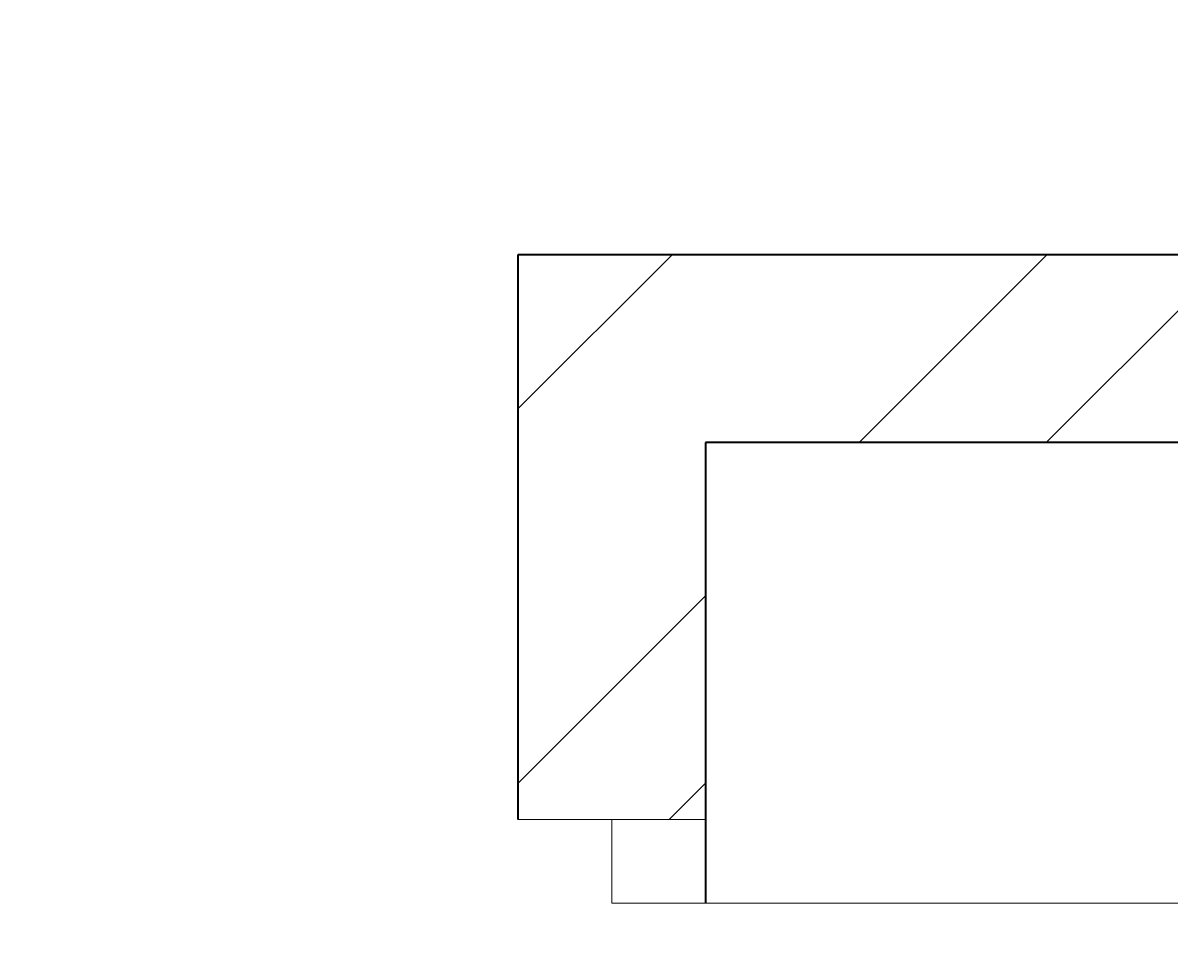
# Model space of a CAD drawing. Units: inches. Extents: x 1962 to 2771, y 1245 to 2660.
# Tile 66 of 114: x 2496 to 2523, y 2113 to 2135. Entities that reach past the tile are written whole.
import ezdxf

# ---------------------------------------------------------------- set-up
doc = ezdxf.new("R2010")
doc.units = ezdxf.units.IN
for name, color, linetype, lineweight in [('A-ANNO-DIMS', 2, 'Continuous', 18), ('A-DOOR', 3, 'Continuous', 18), ('A-WALL', 7, 'Continuous', 35), ('A-WALL-PATT', 252, 'Continuous', 13)]:
    doc.layers.add(name, color=color, linetype=linetype, lineweight=lineweight)
doc.styles.get("Standard").update_dxf_attribs({"font": 'arial.ttf'})
doc.dimstyles.get("Standard").update_dxf_attribs({"dimtxt": 0.18, "dimasz": 0.18, "dimexe": 0.18, "dimexo": 0.0625, "dimgap": 0.09, "dimtad": 0, "dimtih": 1, "dimtoh": 1, "dimdec": 4, "dimzin": 0, "dimdsep": 46, "dimtxsty": 'Standard', "dimcen": 0.09, "dimadec": 0, "dimazin": 0, "dimtfac": 1, "dimtdec": 4, "dimtofl": 0, "dimtmove": 0, "dimatfit": 3, "dimfxl": 1, "dimtolj": 1, "dimtzin": 0, "dimarcsym": 0})

# ---------------------------------------------------------------- blocks, each defined once
blk = doc.blocks.new('*D40')
at = {"layer": 'A-ANNO-DIMS', "color": 0, "lineweight": -2, "transparency": 16777216}
for p, q in [((2072.02, 2033.906), (2072.02, 2583.474)), ((2660.807, 2524.406), (2660.807, 2583.474)), ((2072.2, 2583.294), (2366.02, 2583.294)), ((2660.627, 2583.294), (2366.808, 2583.294))]:
    blk.add_line(p, q, dxfattribs=at)
at = {"layer": 'A-ANNO-DIMS', "color": 0, "transparency": 16777216}
for points in [[(2072.2, 2583.324), (2072.2, 2583.264), (2072.02, 2583.294)], [(2660.627, 2583.324), (2660.627, 2583.264), (2660.807, 2583.294)]]:
    blk.add_solid(points, dxfattribs=at)
at = {"layer": 'Defpoints', "color": 0, "transparency": 16777216}
for p in [(2660.807, 2583.294), (2660.807, 2524.344), (2072.02, 2033.844)]:
    blk.add_point(p, dxfattribs=at)
at = {"layer": 'A-ANNO-DIMS', "color": 0, "transparency": 16777216, "insert": (2366.414, 2583.294), "char_height": 0.18, "attachment_point": 5}
blk.add_mtext('\\A1;588.8', dxfattribs=at)

msp = doc.modelspace()

# ---------------------------------------------------------------- hatches: boundary and pattern name
at = {"layer": 'A-WALL-PATT'}
h = msp.add_hatch(dxfattribs=at)
h.set_pattern_fill('ANSI32', color=256)
h.paths.add_polyline_path([(2090.8074, 2467.3437), (2141.6481, 2467.3437), (2141.6481, 2469.5937), (2141.6481, 2471.8437), (2086.3074, 2471.8437), (2086.3074, 2422.5333), (2090.8074, 2422.5333)])
h.paths.add_polyline_path([(2282.7664, 2471.8437), (2204.8982, 2471.8437), (2204.8982, 2467.3437), (2234.8074, 2467.3437), (2234.8074, 2311.3437), (2228.7492, 2311.3437), (2228.7492, 2306.8437), (2234.8074, 2306.8437), (2331.9227, 2306.8437), (2331.9227, 2309.0937), (2331.9227, 2311.3437), (2239.3074, 2311.3437), (2239.3074, 2467.3437), (2282.7664, 2467.3437), (2282.7664, 2469.5937)])
h.paths.add_polyline_path([(2471.4531, 2519.8437), (2552.011, 2519.8437), (2564.3996, 2519.8437), (2564.3996, 2511.1389), (2568.8996, 2511.1389), (2568.8996, 2524.3437), (2466.9531, 2524.3437), (2466.9531, 2471.8437), (2450.0749, 2471.8437), (2446.4672, 2471.8437), (2446.4672, 2467.3437), (2450.0749, 2467.3437), (2475.9988, 2467.3437), (2475.9988, 2469.5937), (2475.9988, 2471.8437), (2471.4531, 2471.8437)])
h.paths.add_polyline_path([(2575.2231, 2469.5937), (2575.2231, 2471.8437), (2568.8996, 2471.8437), (2568.8996, 2487.1389), (2564.3996, 2487.1389), (2564.3996, 2471.8437), (2556.511, 2471.8437), (2499.2904, 2471.8437), (2499.2904, 2467.3437), (2507.8074, 2467.3437), (2507.8074, 2311.3437), (2414.863, 2311.3437), (2414.863, 2306.8437), (2512.3074, 2306.8437), (2517.0114, 2306.8437), (2517.0114, 2309.0937), (2517.0114, 2311.3437), (2512.3074, 2311.3437), (2512.3074, 2467.3437), (2575.2231, 2467.3437)])
h.paths.add_polyline_path([(2660.8074, 2471.8437), (2600.9602, 2471.8437), (2600.9602, 2467.3437), (2656.3074, 2467.3437), (2656.3074, 2432.5704), (2660.8074, 2432.5704)])
h.paths.add_polyline_path([(2660.8074, 2372.5704), (2656.3074, 2372.5704), (2656.3074, 2311.3437), (2600.276, 2311.3437), (2600.276, 2309.0937), (2600.276, 2306.8437), (2656.3074, 2306.8437), (2656.3074, 2296.2593), (2660.8074, 2296.2593)])
h.paths.add_polyline_path([(2572.3074, 2306.8437), (2577.1385, 2306.8437), (2577.1385, 2311.3437), (2551.082, 2311.3437), (2551.082, 2306.8437), (2567.8074, 2306.8437), (2567.8074, 2258.8437), (2540.0574, 2258.8437), (2540.0574, 2256.5937), (2540.0574, 2254.3437), (2567.8074, 2254.3437), (2656.3074, 2254.3437), (2656.3074, 2236.9085), (2660.8074, 2236.9085), (2660.8074, 2272.2593), (2656.3074, 2272.2593), (2656.3074, 2258.8437), (2572.3074, 2258.8437)])
h.paths.add_polyline_path([(2512.3074, 2254.3437), (2518.8716, 2254.3437), (2518.8716, 2256.5937), (2518.8716, 2258.8437), (2507.8074, 2258.8437), (2507.8074, 2177.8437), (2567.8074, 2177.8437), (2567.8074, 2172.9628), (2572.3074, 2172.9628), (2572.3074, 2177.8437), (2656.3074, 2177.8437), (2656.3074, 2166.4846), (2660.8074, 2166.4846), (2660.8074, 2200.9085), (2656.3074, 2200.9085), (2656.3074, 2182.3437), (2512.3074, 2182.3437)])
h.paths.add_polyline_path([(2656.3074, 2129.8437), (2572.3074, 2129.8437), (2572.3074, 2150.3044), (2570.0574, 2150.3044), (2567.8074, 2150.3044), (2567.8074, 2129.8437), (2507.8074, 2129.8437), (2507.8074, 2116.3027), (2510.0574, 2116.3027), (2512.3074, 2116.3027), (2512.3074, 2125.3437), (2567.8074, 2125.3437), (2572.3074, 2125.3437), (2656.3074, 2125.3437)])
h.paths.add_polyline_path([(2090.8074, 2362.5333), (2086.3074, 2362.5333), (2086.3074, 2298.6242), (2090.8074, 2298.6242), (2090.8074, 2306.8437), (2174.8074, 2306.8437), (2174.8074, 2286.4178), (2179.3074, 2286.4178), (2179.3074, 2306.8437), (2192.8641, 2306.8437), (2192.8641, 2309.0937), (2192.8641, 2311.3437), (2090.8074, 2311.3437)])
h.paths.add_polyline_path([(2209.156, 2258.8437), (2179.3074, 2258.8437), (2179.3074, 2263.2236), (2177.0574, 2263.2236), (2174.8074, 2263.2236), (2174.8074, 2258.8437), (2090.8074, 2258.8437), (2090.8074, 2274.6242), (2086.3074, 2274.6242), (2086.3074, 2238.2967), (2088.5574, 2238.2967), (2090.8074, 2238.2967), (2090.8074, 2254.3437), (2209.156, 2254.3437)])
h.paths.add_polyline_path([(2090.8074, 2177.8437), (2234.8074, 2177.8437), (2234.8074, 2173.1428), (2239.3074, 2173.1428), (2239.3074, 2258.8437), (2230.8442, 2258.8437), (2230.8442, 2256.5937), (2230.8442, 2254.3437), (2234.8074, 2254.3437), (2234.8074, 2182.3437), (2090.8074, 2182.3437), (2090.8074, 2202.2967), (2086.3074, 2202.2967), (2086.3074, 2140.0389), (2090.8074, 2140.0389)])
h.paths.add_polyline_path([(2090.8074, 2080.0389), (2086.3074, 2080.0389), (2086.3074, 2033.8437), (2090.8074, 2033.8437)], flags=17)
h.paths.add_polyline_path([(2244.9405, 2033.8437), (2239.3074, 2033.8437), (2239.3074, 2142.0665), (2237.2592, 2142.0665), (2234.8074, 2142.0665), (2234.8074, 2033.8437), (2090.8074, 2033.8437), (2076.5204, 2033.8437), (2072.0204, 2033.8437), (2072.0204, 2000.4493), (2076.5204, 2000.4493), (2076.5204, 2029.3437), (2090.8074, 2029.3437), (2244.9405, 2029.3437), (2244.9405, 2031.5937)])
h.paths.add_polyline_path([(2234.8074, 1933.3437), (2076.5204, 1933.3437), (2076.5204, 1952.4493), (2074.2704, 1952.4493), (2072.0204, 1952.4493), (2072.0204, 1933.3437), (2072.0204, 1928.8437), (2234.8074, 1928.8437)])
h.paths.add_polyline_path([(2090.8074, 1928.8437), (2086.3074, 1928.8437), (2086.3074, 1906.5013), (2090.8074, 1906.5013)])
h.paths.add_polyline_path([(2090.8074, 1846.5013), (2086.3074, 1846.5013), (2086.3074, 1769.9917), (2088.5574, 1769.9917), (2090.8074, 1769.9917), (2090.8074, 1780.3437), (2234.8074, 1780.3437), (2234.8074, 1708.3437), (2230.3764, 1708.3437), (2230.3764, 1703.8437), (2239.3074, 1703.8437), (2239.3074, 1792.6669), (2237.0574, 1792.6669), (2234.8074, 1792.6669), (2234.8074, 1784.8437), (2090.8074, 1784.8437)])
h.paths.add_polyline_path([(2239.3074, 1928.8437), (2244.9405, 1928.8437), (2244.9405, 1931.0937), (2244.9405, 1933.3437), (2234.8074, 1933.3437), (2234.8074, 1928.8437), (2234.8074, 1825.5949), (2239.3074, 1825.5949)])
h.paths.add_polyline_path([(2148.0425, 1649.0937), (2148.0425, 1651.3437), (2090.8074, 1651.3437), (2090.8074, 1646.8437), (2148.0425, 1646.8437)], flags=0)
h.paths.add_polyline_path([(2207.5601, 1708.3437), (2090.8074, 1708.3437), (2090.8074, 1703.8437), (2174.8074, 1703.8437), (2174.8074, 1651.3437), (2170.4457, 1651.3437), (2170.4457, 1646.8437), (2195.9924, 1646.8437), (2195.9924, 1649.0937), (2195.9924, 1651.3437), (2179.3074, 1651.3437), (2179.3074, 1703.8437), (2207.5601, 1703.8437), (2207.5601, 1706.0937)])
h.paths.add_polyline_path([(2090.8074, 1733.9917), (2086.3074, 1733.9917), (2086.3074, 1696.1032), (2088.5574, 1696.1032), (2090.8074, 1696.1032)])
h.paths.add_polyline_path([(2090.8074, 1672.1032), (2086.3074, 1672.1032), (2086.3074, 1600.3335), (2090.8074, 1600.3335)])
h.paths.add_polyline_path([(2090.8074, 1540.3335), (2086.3074, 1540.3335), (2086.3074, 1486.3437), (2139.6766, 1486.3437), (2139.6766, 1490.8437), (2090.8074, 1490.8437)])
h.paths.add_polyline_path([(2302.3876, 1490.8437), (2239.3074, 1490.8437), (2239.3074, 1646.8437), (2335.9994, 1646.8437), (2335.9994, 1651.3437), (2229.884, 1651.3437), (2229.884, 1646.8437), (2234.8074, 1646.8437), (2234.8074, 1490.8437), (2202.7103, 1490.8437), (2202.7103, 1488.5937), (2202.7103, 1486.3437), (2275.0699, 1486.3437), (2275.0699, 1475.772), (2279.5699, 1475.772), (2279.5699, 1486.3437), (2302.3876, 1486.3437)])
h.paths.add_polyline_path([(2279.5699, 1451.772), (2275.0699, 1451.772), (2275.0699, 1438.3437), (2174.8074, 1438.3437), (2174.8074, 1486.3437), (2179.7922, 1486.3437), (2179.7922, 1490.8437), (2163.3585, 1490.8437), (2163.3585, 1488.5937), (2163.3585, 1486.3437), (2170.3074, 1486.3437), (2170.3074, 1433.8437), (2279.5699, 1433.8437)])
h.paths.add_polyline_path([(2427.2363, 1490.8437), (2375.8074, 1490.8437), (2375.8074, 1646.8437), (2381.6401, 1646.8437), (2381.6401, 1651.3437), (2365.887, 1651.3437), (2365.887, 1649.0937), (2365.887, 1646.8437), (2371.3074, 1646.8437), (2371.3074, 1490.8437), (2327.5627, 1490.8437), (2327.5627, 1488.5937), (2327.5627, 1486.3437), (2371.3074, 1486.3437), (2371.3074, 1433.8437), (2375.8074, 1433.8437), (2375.8074, 1486.3437), (2427.2363, 1486.3437)])
h.paths.add_polyline_path([(2512.3074, 1646.8437), (2519.4351, 1646.8437), (2519.4351, 1649.0937), (2519.4351, 1651.3437), (2507.8074, 1651.3437), (2416.0063, 1651.3437), (2416.0063, 1649.0937), (2416.0063, 1646.8437), (2507.8074, 1646.8437), (2507.8074, 1490.8437), (2497.0532, 1490.8437), (2497.0532, 1488.5937), (2497.0532, 1486.3437), (2574.9344, 1486.3437), (2574.9344, 1476.0181), (2579.4344, 1476.0181), (2579.4344, 1486.3437), (2584.4872, 1486.3437), (2584.3074, 1490.8437), (2512.3074, 1490.8437)])
h.paths.add_polyline_path([(2470.5091, 1486.3437), (2473.9767, 1486.3437), (2473.9767, 1490.8437), (2449.6605, 1490.8437), (2449.6605, 1488.5937), (2449.6605, 1486.3437), (2466.0091, 1486.3437), (2466.0091, 1433.8437), (2470.5091, 1433.8437), (2579.4344, 1433.8437), (2579.4344, 1452.0181), (2574.9344, 1452.0181), (2574.9344, 1438.3437), (2554.5091, 1438.3437), (2470.5091, 1438.3437)])
h.paths.add_polyline_path([(2656.3074, 1490.8437), (2611.86, 1490.8437), (2611.86, 1486.3437), (2656.3074, 1486.3437)])
h.paths.add_polyline_path([(2660.8074, 1532.7007), (2658.5574, 1532.7007), (2656.3074, 1532.7007), (2656.3074, 1486.3437), (2660.8074, 1486.3437)])
h.paths.add_polyline_path([(2660.8074, 1664.9663), (2656.3074, 1664.9663), (2656.3074, 1651.3437), (2602.2313, 1651.3437), (2602.2313, 1646.8437), (2656.3074, 1646.8437), (2656.3074, 1592.7007), (2660.8074, 1592.7007)])
h.paths.add_polyline_path([(2660.8074, 1724.5221), (2656.3074, 1724.5221), (2656.3074, 1703.8437), (2542.4725, 1703.8437), (2542.4725, 1699.3437), (2567.8074, 1699.3437), (2567.8074, 1651.3437), (2552.7766, 1651.3437), (2552.7766, 1649.0937), (2552.7766, 1646.8437), (2577.2878, 1646.8437), (2577.2878, 1649.0937), (2577.2878, 1651.3437), (2572.3074, 1651.3437), (2572.3074, 1699.3437), (2656.3074, 1699.3437), (2656.3074, 1688.9663), (2660.8074, 1688.9663)])
h.paths.add_polyline_path([(2660.8074, 1880.6524), (2656.3074, 1880.6524), (2656.3074, 1832.8437), (2512.3074, 1832.8437), (2512.3074, 1837.8959), (2507.8074, 1837.8959), (2507.8074, 1828.3437), (2567.8074, 1828.3437), (2567.8074, 1804.3437), (2572.3074, 1804.3437), (2572.3074, 1828.3437), (2656.3074, 1828.3437), (2656.3074, 1818.6778), (2660.8074, 1818.6778)])
h.paths.add_polyline_path([(2660.8074, 1794.6778), (2656.3074, 1794.6778), (2656.3074, 1780.3437), (2572.3074, 1780.3437), (2572.3074, 1783.0303), (2570.0574, 1783.0303), (2567.8074, 1783.0303), (2567.8074, 1780.3437), (2507.8074, 1780.3437), (2507.8074, 1699.3437), (2517.8858, 1699.3437), (2517.8858, 1701.5937), (2517.8858, 1703.8437), (2512.3074, 1703.8437), (2512.3074, 1775.8437), (2656.3074, 1775.8437), (2656.3074, 1760.5221), (2660.8074, 1760.5221)])
h.paths.add_polyline_path([(2660.8074, 1981.3437), (2660.8074, 2020.2808), (2658.5574, 2020.2808), (2656.3074, 2020.2808), (2656.3074, 1981.3437), (2512.3074, 1981.3437), (2512.3074, 2086.6996), (2507.8074, 2086.6996), (2507.8074, 1981.3437), (2375.8074, 1981.3437), (2375.8074, 1986.8505), (2373.5574, 1986.8505), (2371.3074, 1986.8505), (2371.3074, 1973.2607), (2375.8074, 1973.2607), (2375.8074, 1976.8437), (2507.8074, 1976.8437), (2507.8074, 1865.4281), (2510.0574, 1865.4281), (2512.3074, 1865.4281), (2512.3074, 1976.8437), (2660.8074, 1976.8437)])
h.paths.add_polyline_path([(2375.8074, 1940.297), (2373.5574, 1940.297), (2371.3074, 1940.297), (2371.3074, 1933.3437), (2278.4434, 1933.3437), (2278.4434, 1928.8437), (2371.3074, 1928.8437), (2371.3074, 1651.3437), (2375.8074, 1651.3437)])
h.paths.add_polyline_path([(2660.8074, 1976.8437), (2656.3074, 1976.8437), (2656.3074, 1940.6524), (2660.8074, 1940.6524)], flags=17)
h.paths.add_polyline_path([(2660.8074, 2142.4846), (2656.3074, 2142.4846), (2656.3074, 2080.2808), (2660.8074, 2080.2808)])
h.paths.add_polyline_path([(2381.4189, 2311.3437), (2375.8074, 2311.3437), (2375.8074, 2467.3437), (2424.7242, 2467.3437), (2424.7242, 2469.5937), (2424.7242, 2471.8437), (2375.8074, 2471.8437), (2375.8074, 2524.3437), (2371.3074, 2524.3437), (2371.3074, 2471.8437), (2307.2097, 2471.8437), (2307.2097, 2467.3437), (2371.3074, 2467.3437), (2371.3074, 2311.3437), (2366.8901, 2311.3437), (2366.8901, 2306.8437), (2371.3074, 2306.8437), (2371.3074, 2033.8437), (2279.6589, 2033.8437), (2279.6589, 2029.3437), (2371.3074, 2029.3437), (2371.3074, 2014.2598), (2375.8074, 2014.2598), (2375.8074, 2306.8437), (2381.4189, 2306.8437)])
h.paths.add_polyline_path([(2263.3074, 2524.3437), (2170.3074, 2524.3437), (2170.3074, 2519.8437), (2170.3074, 2471.8437), (2165.0312, 2471.8437), (2165.0312, 2467.3437), (2179.6721, 2467.3437), (2179.6721, 2469.5161), (2179.6721, 2471.8437), (2174.8074, 2471.8437), (2174.8074, 2519.8437), (2258.8074, 2519.8437), (2258.8074, 2511.6436), (2263.3074, 2511.6436)])
h.paths.add_polyline_path([(2245.0232, 1361.4123), (2492.9468, 1361.4123), (2492.9468, 1398.505), (2245.0232, 1398.505)], flags=9)
h.paths.add_polyline_path([(2388.1434, 2086.6936), (2425.0704, 2086.6936), (2425.0704, 2105.3509), (2388.1434, 2105.3509)], flags=9)
h.paths.add_polyline_path([(2404.922, 2242.6744), (2445.7337, 2242.6744), (2445.7337, 2261.3318), (2404.922, 2261.3318)], flags=9)
h.paths.add_polyline_path([(2269.4107, 2156.7935), (2306.3378, 2156.7935), (2306.3378, 2175.4508), (2269.4107, 2175.4508)], flags=9)
h.paths.add_polyline_path([(2269.3277, 2233.4343), (2306.2547, 2233.4343), (2306.2547, 2252.0917), (2269.3277, 2252.0917)], flags=9)
h.paths.add_polyline_path([(2431.6052, 2320.6922), (2470.4456, 2320.6922), (2470.4456, 2339.3495), (2431.6052, 2339.3495)], flags=25)
h.paths.add_polyline_path([(2249.6902, 2315.7608), (2288.5306, 2315.7608), (2288.5306, 2334.4182), (2249.6902, 2334.4182)], flags=25)
h.paths.add_polyline_path([(2096.9301, 2314.3181), (2135.7704, 2314.3181), (2135.7704, 2332.9755), (2096.9301, 2332.9755)], flags=25)
h.paths.add_polyline_path([(2134.3475, 2285.7089), (2161.4655, 2285.7089), (2161.4655, 2304.3662), (2134.3475, 2304.3662)], flags=9)
h.paths.add_polyline_path([(2126.5155, 2209.4076), (2159.9227, 2209.4076), (2159.9227, 2228.065), (2126.5155, 2228.065)], flags=25)
h.paths.add_polyline_path([(2110.5753, 2141.5299), (2149.4157, 2141.5299), (2149.4157, 2160.1872), (2110.5753, 2160.1872)], flags=25)
h.paths.add_polyline_path([(2249.8618, 1968.3317), (2286.3966, 1968.3317), (2286.3966, 1986.989), (2249.8618, 1986.989)], flags=9)
h.paths.add_polyline_path([(2395.9507, 1777.0051), (2436.7624, 1777.0051), (2436.7624, 1795.6625), (2395.9507, 1795.6625)], flags=9)
h.paths.add_polyline_path([(2398.5259, 1888.5651), (2435.0062, 1888.5651), (2435.0062, 1907.2224), (2398.5259, 1907.2224)], flags=25)
h.paths.add_polyline_path([(2259.3506, 1728.3559), (2296.2776, 1728.3559), (2296.2776, 1747.0132), (2259.3506, 1747.0132)], flags=9)
h.paths.add_polyline_path([(2271.3698, 1845.268), (2308.2968, 1845.268), (2308.2968, 1863.9253), (2271.3698, 1863.9253)], flags=9)
h.paths.add_polyline_path([(2120.9355, 1786.3027), (2159.7759, 1786.3027), (2159.7759, 1804.9601), (2120.9355, 1804.9601)], flags=25)
h.paths.add_polyline_path([(2121.3164, 1732.1043), (2154.7236, 1732.1043), (2154.7236, 1750.7616), (2121.3164, 1750.7616)], flags=25)
h.paths.add_polyline_path([(2118.3706, 1678.8997), (2147.5282, 1678.8997), (2147.5282, 1697.557), (2118.3706, 1697.557)], flags=25)
h.paths.add_polyline_path([(2385.9227, 1493.557), (2424.763, 1493.557), (2424.763, 1512.2143), (2385.9227, 1512.2143)], flags=25)
h.paths.add_polyline_path([(2248.7058, 1500.0256), (2287.5462, 1500.0256), (2287.5462, 1518.6829), (2248.7058, 1518.6829)], flags=25)
h.paths.add_polyline_path([(2104.1669, 1617.3771), (2143.0073, 1617.3771), (2143.0073, 1636.0344), (2104.1669, 1636.0344)], flags=9)
h.paths.add_polyline_path([(2096.0714, 1447.8824), (2137.3845, 1447.8824), (2137.3845, 1458.1859), (2096.0714, 1458.1859)], flags=9)
h.paths.add_polyline_path([(2180.6114, 1440.325), (2209.7689, 1440.325), (2209.7689, 1458.9823), (2180.6114, 1458.9823)], flags=25)
h.paths.add_polyline_path([(2316.1698, 1447.9637), (2357.4829, 1447.9637), (2357.4829, 1458.2673), (2316.1698, 1458.2673)], flags=9)
h.paths.add_polyline_path([(2397.6187, 1447.9637), (2438.9318, 1447.9637), (2438.9318, 1458.2673), (2397.6187, 1458.2673)], flags=9)
h.paths.add_polyline_path([(2473.0778, 1439.5953), (2502.2354, 1439.5953), (2502.2354, 1458.2527), (2473.0778, 1458.2527)], flags=25)
h.paths.add_polyline_path([(2589.7027, 1447.8819), (2631.0158, 1447.8819), (2631.0158, 1458.1855), (2589.7027, 1458.1855)], flags=9)
h.paths.add_polyline_path([(2522.4009, 1497.5285), (2561.2413, 1497.5285), (2561.2413, 1516.1859), (2522.4009, 1516.1859)], flags=25)
h.paths.add_polyline_path([(2579.6565, 1671.3482), (2608.8141, 1671.3482), (2608.8141, 1690.0056), (2579.6565, 1690.0056)], flags=25)
h.paths.add_polyline_path([(2544.7038, 1725.5064), (2578.1111, 1725.5064), (2578.1111, 1744.1637), (2544.7038, 1744.1637)], flags=25)
h.paths.add_polyline_path([(2578.1191, 1807.472), (2607.2766, 1807.472), (2607.2766, 1826.1293), (2578.1191, 1826.1293)], flags=25)
h.paths.add_polyline_path([(2595.0614, 1835.1839), (2633.9018, 1835.1839), (2633.9018, 1853.8413), (2595.0614, 1853.8413)], flags=25)
h.paths.add_polyline_path([(2567.0097, 2097.7035), (2605.8501, 2097.7035), (2605.8501, 2116.3609), (2567.0097, 2116.3609)], flags=9)
h.paths.add_polyline_path([(2586.644, 2134.6454), (2615.8015, 2134.6454), (2615.8015, 2153.3027), (2586.644, 2153.3027)], flags=9)
h.paths.add_polyline_path([(2544.6185, 2212.6783), (2578.0258, 2212.6783), (2578.0258, 2231.3356), (2544.6185, 2231.3356)], flags=25)
h.paths.add_polyline_path([(2577.0273, 2256.9023), (2606.1849, 2256.9023), (2606.1849, 2275.5597), (2577.0273, 2275.5597)], flags=24)
h.paths.add_polyline_path([(2605.2683, 2315.2821), (2644.1087, 2315.2821), (2644.1087, 2333.9395), (2605.2683, 2333.9395)], flags=25)
h.paths.add_polyline_path([(2583.1244, 2496.1815), (2624.4375, 2496.1815), (2624.4375, 2506.4851), (2583.1244, 2506.4851)], flags=9)
h.paths.add_polyline_path([(2474.761, 2497.0823), (2503.9185, 2497.0823), (2503.9185, 2515.7397), (2474.761, 2515.7397)], flags=25)
h.paths.add_polyline_path([(2387.5787, 2494.2563), (2428.902, 2494.2563), (2428.902, 2504.5598), (2387.5787, 2504.5598)], flags=9)
h.paths.add_polyline_path([(2300.1657, 2500.1564), (2341.4788, 2500.1564), (2341.4788, 2510.46), (2300.1657, 2510.46)], flags=25)
h.paths.add_polyline_path([(2176.8589, 2497.5843), (2206.0165, 2497.5843), (2206.0165, 2516.2416), (2176.8589, 2516.2416)], flags=25)
h.paths.add_polyline_path([(2097.4668, 2494.9762), (2138.7799, 2494.9762), (2138.7799, 2505.2798), (2097.4668, 2505.2798)], flags=9)

# ---------------------------------------------------------------- linework, layer by layer
at = {"layer": 'A-DOOR'}
for p, q in [((2512.3074, 2116.3027), (2507.8074, 2116.3027)), ((2507.8074, 2116.3027), (2510.0574, 2116.3027)), ((2510.0574, 2116.3027), (2510.0574, 2114.3027)), ((2510.0574, 2114.3027), (2546.0574, 2114.3027))]:
    msp.add_line(p, q, dxfattribs=at)
msp.add_arc((2518.9529, 2114.3027), 27.1044, 250.84069, 360, dxfattribs=at)
at = {"layer": 'A-WALL'}
for p, q in [((2567.8074, 2129.8437), (2507.8074, 2129.8437)), ((2507.8074, 2129.8437), (2507.8074, 2116.3027)), ((2507.8074, 2125.3437), (2507.8074, 2116.3027)), ((2512.3074, 2125.3437), (2512.3074, 2114.3027)), ((2567.8074, 2125.3437), (2512.3074, 2125.3437))]:
    msp.add_line(p, q, dxfattribs=at)

# ---------------------------------------------------------------- dimensions: what is measured, and where the dimension line sits
at = {"layer": 'A-ANNO-DIMS'}
dim = msp.add_linear_dim(base=(2660.8074, 2583.2937), p1=(2072.0204, 2033.8437), p2=(2660.8074, 2524.3437), dimstyle='Standard', override={"dimdec": 1, "dimlfac": 1, "dimrnd": 0, "dimzin": 0, "dimdsep": 46, "dimlunit": 2}, dxfattribs=at)
dim.commit()
dim.dimension.update_dxf_attribs({"geometry": '*D40', "text_midpoint": (2366.4139, 2583.2937)})

doc.saveas('drawing.dxf')
